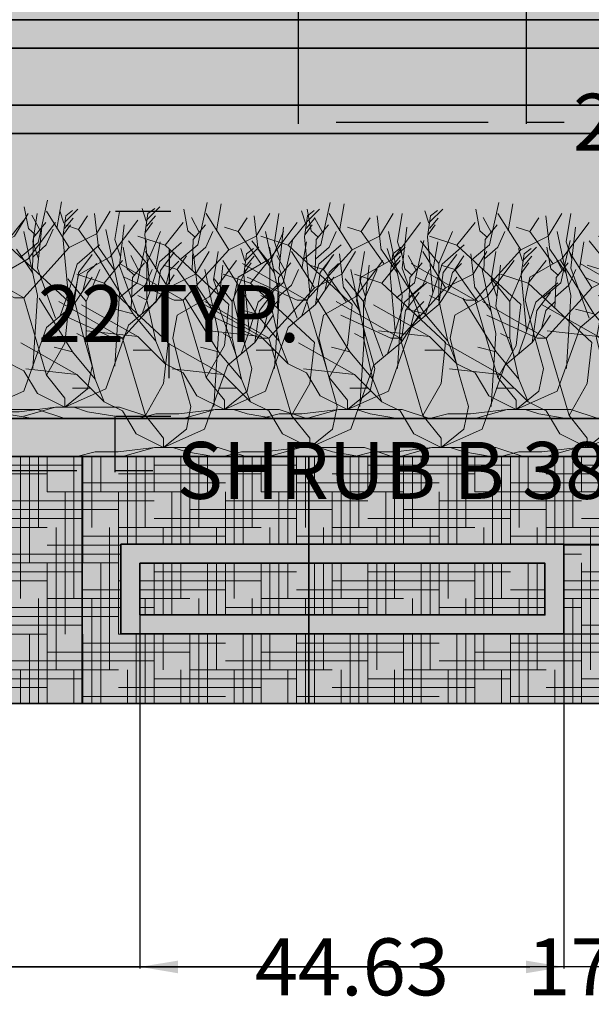
# Model space of a CAD drawing. Units: inches. Extents: x 221 to 874, y 171 to 738.
# Tile 7 of 11: x 650 to 710, y 171 to 275. Entities that reach past the tile are written whole.
import ezdxf

# ---------------------------------------------------------------- set-up
doc = ezdxf.new("R2010")
doc.units = ezdxf.units.IN
doc.header["$MEASUREMENT"] = 0
for name, color, linetype, lineweight in [('A-ANNO-DIMS', 2, 'Continuous', 18), ('A-ELEV', 7, 'Continuous', 35), ('A-ELEV-PATT', 8, 'Continuous', 13), ('L-PLNT', 3, 'Continuous', 13)]:
    doc.layers.add(name, color=color, linetype=linetype, lineweight=lineweight)
doc.styles.get("Standard").update_dxf_attribs({"font": 'arial.ttf'})
doc.dimstyles.get("Standard").update_dxf_attribs({"dimtxt": 6, "dimasz": 4, "dimexe": 0.18, "dimexo": 0.0625, "dimgap": 0.09, "dimtad": 0, "dimtih": 1, "dimtoh": 1, "dimdec": 0, "dimzin": 0, "dimdsep": 46, "dimlunit": 3, "dimtxsty": 'Standard', "dimcen": 0.09, "dimadec": 0, "dimazin": 0, "dimtfac": 1, "dimtdec": 0, "dimtofl": 0, "dimtmove": 0, "dimatfit": 3, "dimfxl": 1, "dimtolj": 1, "dimtzin": 0, "dimarcsym": 0})

# ---------------------------------------------------------------- blocks, each defined once
blk = doc.blocks.new('SHRUB-A')
for p, q in [((15.5, 17.76), (13.1, 21.6)), ((18.38, 19.2), (19.82, 21.6)), ((8.78, 18.24), (10.7, 20.64)), ((19.82, 16.8), (22.7, 20.64)), ((6.86, 16.32), (4.94, 18.72)), ((8.78, 18.24), (5.9, 19.2)), ((6.86, 16.32), (8.3, 19.68)), ((15.5, 17.76), (18.38, 19.2)), ((15.5, 12), (8.78, 18.24)), ((10.7, 12.48), (15.5, 17.76)), ((5.42, 11.04), (1.91, 16.66)), ((16.46, 14.88), (19.82, 16.8)), ((25.1, 15.36), (26.54, 17.28)), ((10.7, 12.48), (3.98, 16.32)), ((6.86, 12.48), (6.86, 16.32)), ((9.74, 12.48), (4.46, 14.88)), ((15.98, 12.48), (16.46, 14.88)), ((24.62, 12), (25.1, 15.36)), ((24.62, 12), (26.54, 14.88)), ((6.86, 12.48), (5.9, 12.96)), ((7.82, 8.16), (6.86, 12.48)), ((10.7, 12.48), (9.74, 12.48)), ((13.1, 4.32), (10.7, 12.48)), ((16.94, 8.64), (15.98, 12.48)), ((5.9, 8.64), (0, 11.96)), ((5.42, 11.04), (3.5, 11.52)), ((15.02, 7.68), (15.5, 12)), ((21.74, 9.6), (24.62, 12)), ((7.82, 8.16), (5.42, 11.04)), ((19.34, 2.88), (21.74, 9.6)), ((5.9, 8.64), (0.53, 9.22)), ((8.78, 5.76), (5.9, 8.64)), ((17.9, 5.28), (16.94, 8.64)), ((8.78, 5.76), (7.82, 8.16)), ((13.1, 4.32), (15.02, 7.68)), ((10.7, 4.8), (8.78, 5.76)), ((17.42, 2.88), (17.9, 5.28)), ((12.14, 2.4), (10.7, 4.8)), ((15.02, 1.92), (13.1, 4.32)), ((15.02, 0.96), (12.14, 2.4)), ((15.02, 0.96), (19.34, 2.88)), ((15.02, 0.96), (17.42, 2.88)), ((15.02, 0.96), (15.02, 1.92)), ((15.02, 0.96), (20.78, 0.96)), ((20.78, 0.96), (23.66, 0))]:
    blk.add_line(p, q)
blk = doc.blocks.new('GRASS-TUFT')
for p, q in [((0.28, 8.35), (0.58, 10.54)), ((0.58, 10.54), (1.31, 11.09)), ((0.83, 2.4), (0.28, 8.35)), ((1.8, 5.45), (4.12, 7.49)), ((0.83, 2.4), (1.8, 5.45)), ((0, 0), (0.83, 2.4))]:
    blk.add_line(p, q)
blk = doc.blocks.new('SHRUB-B')
for p, q in [((15.5, 17.76), (13.1, 21.6)), ((18.38, 19.2), (19.82, 21.6)), ((8.78, 18.24), (10.7, 20.64)), ((19.82, 16.8), (22.7, 20.64)), ((6.86, 16.32), (4.94, 18.72)), ((8.78, 18.24), (5.9, 19.2)), ((6.86, 16.32), (8.3, 19.68)), ((15.5, 17.76), (18.38, 19.2)), ((15.5, 12), (8.78, 18.24)), ((10.7, 12.48), (15.5, 17.76)), ((5.42, 11.04), (1.91, 16.66)), ((16.46, 14.88), (19.82, 16.8)), ((25.1, 15.36), (26.54, 17.28)), ((10.7, 12.48), (3.98, 16.32)), ((6.86, 12.48), (6.86, 16.32)), ((9.74, 12.48), (4.46, 14.88)), ((15.98, 12.48), (16.46, 14.88)), ((24.62, 12), (25.1, 15.36)), ((24.62, 12), (26.54, 14.88)), ((6.86, 12.48), (5.9, 12.96)), ((7.82, 8.16), (6.86, 12.48)), ((10.7, 12.48), (9.74, 12.48)), ((13.1, 4.32), (10.7, 12.48)), ((16.94, 8.64), (15.98, 12.48)), ((5.9, 8.64), (0, 11.96)), ((5.42, 11.04), (3.5, 11.52)), ((15.02, 7.68), (15.5, 12)), ((21.74, 9.6), (24.62, 12)), ((7.82, 8.16), (5.42, 11.04)), ((19.34, 2.88), (21.74, 9.6)), ((5.9, 8.64), (0.53, 9.22)), ((8.78, 5.76), (5.9, 8.64)), ((17.9, 5.28), (16.94, 8.64)), ((8.78, 5.76), (7.82, 8.16)), ((13.1, 4.32), (15.02, 7.68)), ((10.7, 4.8), (8.78, 5.76)), ((17.42, 2.88), (17.9, 5.28)), ((12.14, 2.4), (10.7, 4.8)), ((15.02, 1.92), (13.1, 4.32)), ((15.02, 0.96), (12.14, 2.4)), ((15.02, 0.96), (19.34, 2.88)), ((15.02, 0.96), (17.42, 2.88)), ((15.02, 0.96), (15.02, 1.92)), ((15.02, 0.96), (20.78, 0.96)), ((20.78, 0.96), (23.66, 0)), ((25.58, 0.48), (23.66, 0)), ((27.98, 0.48), (25.58, 0.48)), ((31.82, 0.96), (27.98, 0.48)), ((31.82, 0.96), (28.46, 0)), ((31.82, 0.96), (33.74, 0.96)), ((33.74, 0.96), (35.18, 0.48)), ((35.18, 0.48), (38.06, 0))]:
    blk.add_line(p, q)
blk = doc.blocks.new('GRASS-SPRIG')
for p, q in [((1.44, 3.36), (2.4, 4.8)), ((1.44, 3.36), (0, 3.84)), ((3.84, 0), (1.44, 3.36))]:
    blk.add_line(p, q)
blk = doc.blocks.new('*D13')
at = {"layer": 'A-ANNO-DIMS', "color": 0, "lineweight": -2, "transparency": 16777216}
for p, q in [((678.91, 283.65), (678.91, 263.74)), ((702.91, 283.65), (702.91, 263.74)), ((682.91, 263.92), (698.91, 263.92)), ((702.91, 263.92), (706.91, 263.92))]:
    blk.add_line(p, q, dxfattribs=at)
at = {"layer": 'A-ANNO-DIMS', "color": 0, "transparency": 16777216}
for points in [[(682.91, 264.58), (682.91, 263.25), (678.91, 263.92)], [(698.91, 264.58), (698.91, 263.25), (702.91, 263.92)]]:
    blk.add_solid(points, dxfattribs=at)
at = {"layer": 'Defpoints', "color": 0, "transparency": 16777216}
for p in [(678.91, 283.72), (702.91, 283.72), (702.91, 263.92)]:
    blk.add_point(p, dxfattribs=at)
at = {"layer": 'A-ANNO-DIMS', "color": 0, "transparency": 16777216, "insert": (721.65, 263.92), "char_height": 6, "attachment_point": 5}
blk.add_mtext('\\A1;24 TYP.', dxfattribs=at)
blk = doc.blocks.new('*D16')
at = {"layer": 'A-ANNO-DIMS', "color": 0, "lineweight": -2, "transparency": 16777216}
for p, q in [((621.56, 232.89), (621.56, 227.07)), ((659.62, 232.89), (659.62, 227.07)), ((625.56, 227.25), (655.62, 227.25)), ((659.62, 227.25), (663.62, 227.25))]:
    blk.add_line(p, q, dxfattribs=at)
at = {"layer": 'A-ANNO-DIMS', "color": 0, "transparency": 16777216}
for points in [[(625.56, 227.91), (625.56, 226.58), (621.56, 227.25)], [(655.62, 227.91), (655.62, 226.58), (659.62, 227.25)]]:
    blk.add_solid(points, dxfattribs=at)
at = {"layer": 'Defpoints', "color": 0, "transparency": 16777216}
for p in [(621.56, 232.96), (659.62, 232.96), (659.62, 227.25)]:
    blk.add_point(p, dxfattribs=at)
at = {"layer": 'A-ANNO-DIMS', "color": 0, "transparency": 16777216, "insert": (698.1, 227.25), "char_height": 6, "attachment_point": 5}
blk.add_mtext('\\A1;SHRUB B 38 TYP.', dxfattribs=at)
blk = doc.blocks.new('*D17')
at = {"layer": 'A-ANNO-DIMS', "color": 0, "lineweight": -2, "transparency": 16777216}
for p, q in [((659.69, 254.56), (665.51, 254.56)), ((665.33, 250.56), (665.33, 246.86)), ((665.33, 236.96), (665.33, 240.65)), ((659.69, 232.96), (665.51, 232.96))]:
    blk.add_line(p, q, dxfattribs=at)
at = {"layer": 'A-ANNO-DIMS', "color": 0, "transparency": 16777216}
for points in [[(664.67, 250.56), (666, 250.56), (665.33, 254.56)], [(664.67, 236.96), (666, 236.96), (665.33, 232.96)]]:
    blk.add_solid(points, dxfattribs=at)
at = {"layer": 'Defpoints', "color": 0, "transparency": 16777216}
for p in [(659.62, 254.56), (665.33, 254.56), (659.62, 232.96)]:
    blk.add_point(p, dxfattribs=at)
at = {"layer": 'A-ANNO-DIMS', "color": 0, "transparency": 16777216, "insert": (665.33, 243.76), "char_height": 6, "attachment_point": 5}
blk.add_mtext('\\A1;22 TYP.', dxfattribs=at)
blk = doc.blocks.new('*D20')
at = {"layer": 'A-ANNO-DIMS', "color": 0, "lineweight": -2, "transparency": 16777216}
for p, q in [((313.08, 202.65), (313.08, 174.79)), ((805.08, 202.65), (805.08, 174.79)), ((317.08, 174.97), (552.27, 174.97)), ((801.08, 174.97), (565.89, 174.97))]:
    blk.add_line(p, q, dxfattribs=at)
at = {"layer": 'A-ANNO-DIMS', "color": 0, "transparency": 16777216}
for points in [[(317.08, 175.63), (317.08, 174.3), (313.08, 174.97)], [(801.08, 175.63), (801.08, 174.3), (805.08, 174.97)]]:
    blk.add_solid(points, dxfattribs=at)
at = {"layer": 'Defpoints', "color": 0, "transparency": 16777216}
for p in [(313.08, 202.72), (805.08, 202.72), (805.08, 174.97)]:
    blk.add_point(p, dxfattribs=at)
at = {"layer": 'A-ANNO-DIMS', "color": 0, "transparency": 16777216, "insert": (559.08, 174.97), "char_height": 6, "attachment_point": 5}
blk.add_mtext('\\A1;492', dxfattribs=at)
blk = doc.blocks.new('*D21')
at = {"layer": 'A-ANNO-DIMS', "color": 0, "lineweight": -2, "transparency": 16777216}
for p, q in [((541.14, 706.72), (833.01, 706.72)), ((832.83, 702.72), (832.83, 457.87)), ((832.83, 206.72), (832.83, 451.56)), ((805.14, 202.72), (833.01, 202.72))]:
    blk.add_line(p, q, dxfattribs=at)
at = {"layer": 'A-ANNO-DIMS', "color": 0, "transparency": 16777216}
for points in [[(832.16, 702.72), (833.5, 702.72), (832.83, 706.72)], [(832.16, 206.72), (833.5, 206.72), (832.83, 202.72)]]:
    blk.add_solid(points, dxfattribs=at)
at = {"layer": 'Defpoints', "color": 0, "transparency": 16777216}
for p in [(541.08, 706.72), (832.83, 706.72), (805.08, 202.72)]:
    blk.add_point(p, dxfattribs=at)
at = {"layer": 'A-ANNO-DIMS', "color": 0, "transparency": 16777216, "insert": (832.83, 454.72), "char_height": 6, "attachment_point": 5}
blk.add_mtext('\\A1;504', dxfattribs=at)
blk = doc.blocks.new('*D64')
at = {"layer": 'A-ANNO-DIMS', "color": 0, "lineweight": -2, "transparency": 16777216}
for p, q in [((832.83, 284.72), (832.83, 288.72)), ((832.83, 288.72), (836.83, 288.72)), ((705.97, 280.72), (833.01, 280.72)), ((781.14, 274.72), (833.01, 274.72)), ((832.83, 270.72), (832.83, 266.72))]:
    blk.add_line(p, q, dxfattribs=at)
at = {"layer": 'A-ANNO-DIMS', "color": 0, "transparency": 16777216}
for points in [[(832.16, 284.72), (833.5, 284.72), (832.83, 280.72)], [(832.16, 270.72), (833.5, 270.72), (832.83, 274.72)]]:
    blk.add_solid(points, dxfattribs=at)
at = {"layer": 'Defpoints', "color": 0, "transparency": 16777216}
for p in [(705.91, 280.72), (832.83, 280.72), (781.08, 274.72)]:
    blk.add_point(p, dxfattribs=at)
at = {"layer": 'A-ANNO-DIMS', "color": 0, "transparency": 16777216, "insert": (838.9, 288.72), "char_height": 6, "attachment_point": 5}
blk.add_mtext('\\A1;6', dxfattribs=at)
blk = doc.blocks.new('*D70')
at = {"layer": 'A-ANNO-DIMS', "color": 0, "lineweight": -2, "transparency": 16777216}
for p, q in [((625.96, 229.65), (625.96, 174.79)), ((805.08, 202.65), (805.08, 174.79)), ((629.96, 174.97), (703.29, 174.97)), ((801.08, 174.97), (727.75, 174.97))]:
    blk.add_line(p, q, dxfattribs=at)
at = {"layer": 'A-ANNO-DIMS', "color": 0, "transparency": 16777216}
for points in [[(629.96, 175.63), (629.96, 174.3), (625.96, 174.97)], [(801.08, 175.63), (801.08, 174.3), (805.08, 174.97)]]:
    blk.add_solid(points, dxfattribs=at)
at = {"layer": 'Defpoints', "color": 0, "transparency": 16777216}
for p in [(625.96, 229.72), (805.08, 202.72), (805.08, 174.97)]:
    blk.add_point(p, dxfattribs=at)
at = {"layer": 'A-ANNO-DIMS', "color": 0, "transparency": 16777216, "insert": (715.52, 174.97), "char_height": 6, "attachment_point": 5}
blk.add_mtext('\\A1;179.12', dxfattribs=at)
blk = doc.blocks.new('*D71')
at = {"layer": 'A-ANNO-DIMS', "color": 0, "lineweight": -2, "transparency": 16777216}
for p, q in [((662.26, 211.97), (662.26, 174.79)), ((706.89, 209.97), (706.89, 174.79)), ((666.26, 174.97), (674.24, 174.97)), ((702.89, 174.97), (694.91, 174.97))]:
    blk.add_line(p, q, dxfattribs=at)
at = {"layer": 'A-ANNO-DIMS', "color": 0, "transparency": 16777216}
for points in [[(666.26, 175.63), (666.26, 174.3), (662.26, 174.97)], [(702.89, 175.63), (702.89, 174.3), (706.89, 174.97)]]:
    blk.add_solid(points, dxfattribs=at)
at = {"layer": 'Defpoints', "color": 0, "transparency": 16777216}
for p in [(662.26, 212.04), (706.89, 210.04), (706.89, 174.97)]:
    blk.add_point(p, dxfattribs=at)
at = {"layer": 'A-ANNO-DIMS', "color": 0, "transparency": 16777216, "insert": (684.57, 174.97), "char_height": 6, "attachment_point": 5}
blk.add_mtext('\\A1;44.63', dxfattribs=at)
blk = doc.blocks.new('*D72')
at = {"layer": 'A-ANNO-DIMS', "color": 0, "lineweight": -2, "transparency": 16777216}
for p, q in [((832.83, 219.48), (832.83, 223.48)), ((832.83, 223.48), (836.83, 223.48)), ((706.95, 219.48), (833.01, 219.48)), ((832.83, 214.04), (832.83, 215.48)), ((706.95, 210.04), (833.01, 210.04))]:
    blk.add_line(p, q, dxfattribs=at)
at = {"layer": 'A-ANNO-DIMS', "color": 0, "transparency": 16777216}
for points in [[(832.16, 215.48), (833.5, 215.48), (832.83, 219.48)], [(832.16, 214.04), (833.5, 214.04), (832.83, 210.04)]]:
    blk.add_solid(points, dxfattribs=at)
at = {"layer": 'Defpoints', "color": 0, "transparency": 16777216}
for p in [(706.89, 219.48), (832.83, 219.48), (706.89, 210.04)]:
    blk.add_point(p, dxfattribs=at)
at = {"layer": 'A-ANNO-DIMS', "color": 0, "transparency": 16777216, "insert": (847.03, 223.48), "char_height": 6, "attachment_point": 5}
blk.add_mtext('\\A1;9.444', dxfattribs=at)

msp = doc.modelspace()

# ---------------------------------------------------------------- hatches: boundary and pattern name
at = {"layer": 'A-ELEV-PATT'}
h = msp.add_hatch(color=256, dxfattribs=at)
h.dxf.hatch_style = 1
h.paths.add_polyline_path([(349.0786, 286.1996), (313.0786, 286.1996), (313.0786, 232.7164), (349.0786, 232.7164)])
h.paths.add_polyline_path([(464.0786, 286.1996), (406.0786, 286.1996), (406.0786, 232.7164), (464.0786, 232.7164)])
h.paths.add_polyline_path([(541.0786, 286.1996), (493.0786, 286.1996), (493.0786, 232.7164), (541.0786, 232.7164)])
h.paths.add_polyline_path([(541.0786, 370.7164), (493.0786, 370.7164), (493.0786, 286.1996), (541.0786, 286.1996)])
h.paths.add_polyline_path([(464.0786, 370.7164), (406.0786, 370.7164), (406.0786, 286.1996), (464.0786, 286.1996)])
h.paths.add_polyline_path([(349.0786, 370.7164), (313.0786, 370.7164), (313.0786, 286.1996), (349.0786, 286.1996)])
h.paths.add_polyline_path([(349.0786, 454.7164), (313.0786, 454.7164), (313.0786, 370.7164), (349.0786, 370.7164)])
h.paths.add_polyline_path([(464.0786, 454.7164), (406.0786, 454.7164), (406.0786, 370.7164), (464.0786, 370.7164)])
h.paths.add_polyline_path([(541.0786, 418.7164), (541.0786, 454.7164), (493.0786, 454.7164), (493.0786, 370.7164), (541.0786, 370.7164)])
h.paths.add_polyline_path([(541.0786, 550.7164), (493.0786, 550.7164), (493.0786, 454.7164), (541.0786, 454.7164)])
h.paths.add_polyline_path([(464.0786, 550.7164), (406.0786, 550.7164), (406.0786, 454.7164), (464.0786, 454.7164)])
h.paths.add_polyline_path([(349.0786, 550.7164), (313.0786, 550.7164), (313.0786, 454.7164), (349.0786, 454.7164)])
h.paths.add_polyline_path([(349.0786, 586.7164), (313.0786, 586.7164), (313.0786, 550.7164), (349.0786, 550.7164)])
h.paths.add_polyline_path([(464.0786, 586.7164), (406.0786, 586.7164), (406.0786, 550.7164), (464.0786, 550.7164)])
h.paths.add_polyline_path([(541.0786, 574.7164), (541.0786, 586.7164), (493.0786, 586.7164), (493.0786, 550.7164), (541.0786, 550.7164)])
h.paths.add_polyline_path([(541.0786, 670.7164), (493.0786, 670.7164), (493.0786, 586.7164), (541.0786, 586.7164)])
h.paths.add_polyline_path([(464.0786, 670.7164), (406.0786, 670.7164), (406.0786, 586.7164), (464.0786, 586.7164)])
h.paths.add_polyline_path([(349.0786, 670.7164), (313.0786, 670.7164), (313.0786, 586.7164), (349.0786, 586.7164)])
h.paths.add_polyline_path([(406.0786, 706.7164), (313.0786, 706.7164), (313.0786, 670.7164), (349.0786, 670.7164), (406.0786, 670.7164)])
h.paths.add_polyline_path([(464.0786, 706.7164), (406.0786, 706.7164), (406.0786, 670.7164), (464.0786, 670.7164)])
h.paths.add_polyline_path([(541.0786, 706.7164), (493.0786, 706.7164), (493.0786, 688.7164), (493.0786, 670.7164), (541.0786, 670.7164)])
h.paths.add_polyline_path([(660.0786, 610.7164), (541.0786, 610.7164), (541.0786, 586.7164), (541.0786, 574.7164), (660.0786, 574.7164)])
h.paths.add_polyline_path([(781.0786, 610.7164), (660.0786, 610.7164), (660.0786, 574.7164), (769.0786, 574.7164), (781.0786, 574.7164)])
h.paths.add_polyline_path([(781.0786, 574.7164), (769.0786, 574.7164), (769.0786, 476.1199), (781.0786, 476.1199)])
h.paths.add_polyline_path([(781.0786, 476.1199), (769.0786, 476.1199), (769.0786, 457.7164), (781.0786, 457.7164)])
h.paths.add_polyline_path([(781.0786, 377.1023), (705.9097, 377.1023), (705.9097, 286.1996), (781.0786, 286.1996)])
h.paths.add_polyline_path([(741.9618, 338.8486), (756.9618, 338.8486), (756.9618, 329.8486), (741.9618, 329.8486)], flags=16)
h.paths.add_polyline_path([(648.9097, 377.1023), (598.0786, 377.1023), (598.0786, 286.1996), (648.9097, 286.1996)])
h.paths.add_polyline_path([(781.0786, 286.1996), (705.9097, 286.1996), (705.9097, 280.7164), (648.9097, 280.7164), (648.9097, 286.1996), (598.0786, 286.1996), (598.0786, 280.7164), (550.0786, 280.7164), (550.0786, 286.1996), (541.0786, 286.1996), (541.0786, 274.7164), (781.0786, 274.7164)])
h.paths.add_polyline_path([(660.0786, 562.7164), (546.3477, 562.7164), (546.3477, 457.7164), (660.0786, 457.7164)])
h = msp.add_hatch(color=256, dxfattribs=at)
h.set_gradient(color1=(99, 100, 102), color2=(169, 160, 132), name='INVCYLINDER')
h.paths.add_polyline_path([(541.0786, 274.7164), (541.0786, 271.7164), (787.0786, 271.7164), (781.0786, 274.7164)])
h = msp.add_hatch(color=256, dxfattribs=at)
h.paths.add_polyline_path([(787.0786, 271.7164), (541.0786, 271.7164), (541.0786, 265.7164), (799.0786, 265.7164)])
h.paths.add_polyline_path([(631.9596, 262.7164), (541.0786, 262.7164), (541.0786, 256.7164), (631.9596, 256.7164)])
h.paths.add_polyline_path([(631.9596, 253.7164), (541.0786, 253.7164), (541.0786, 247.7164), (631.9596, 247.7164)])
h.paths.add_polyline_path([(631.9596, 244.7164), (541.0786, 244.7164), (541.0786, 238.7164), (631.9596, 238.7164)])
h.paths.add_polyline_path([(631.9596, 235.7164), (541.0786, 235.7164), (541.0786, 229.7164), (625.9596, 229.7164), (625.9596, 232.7164), (631.9596, 232.7164)])
h.paths.add_polyline_path([(630.2472, 217.7164), (538.2859, 217.7164), (538.2859, 211.7164), (634.5124, 211.7164), (634.5123, 211.7326)], flags=17)
h.paths.add_polyline_path([(634.5396, 208.7164), (538.2859, 208.7164), (538.2859, 202.7164), (638.8162, 202.7164)])
h = msp.add_hatch(color=256, dxfattribs=at)
h.set_gradient(color1=(99, 100, 102), color2=(248, 246, 176), name='CYLINDER')
h.paths.add_polyline_path([(805.0786, 262.7164), (799.0786, 265.7164), (541.0786, 265.7164), (541.0786, 262.7164)])
for points in [[(631.9596, 262.7164), (631.9596, 232.7164), (805.0786, 232.7164), (805.0786, 262.7164)], [(805.0786, 228.7164), (805.0786, 232.7164), (625.9596, 232.7164), (625.9596, 228.7164)]]:
    msp.add_hatch(color=256, dxfattribs=at).paths.add_polyline_path(points)
h = msp.add_hatch(color=256, dxfattribs=at)
h.set_gradient(color1=(147, 149, 152), color2=(99, 100, 102), name='CURVED')
h.paths.add_polyline_path([(656.1863, 228.7164), (625.9606, 228.7164), (625.9626, 226.7164), (630.2279, 220.7164), (630.2471, 217.7164), (634.5238, 211.7164), (634.5124, 211.7164), (634.5315, 208.7276), (638.8162, 202.7164), (656.1863, 202.7164)])
h = msp.add_hatch(dxfattribs=at)
h.set_pattern_fill('HOUND', color=256, scale=15, style=0)
h.paths.add_polyline_path([(656.1863, 228.7164), (625.9606, 228.7164), (625.9626, 226.7164), (630.2279, 220.7164), (630.2471, 217.7164), (634.5238, 211.7164), (634.5124, 211.7164), (634.5315, 208.7276), (638.8162, 202.7164), (656.1863, 202.7164)])
h = msp.add_hatch(color=256, dxfattribs=at)
h.set_gradient(color1=(99, 100, 102), color2=(91, 91, 91), rotation=180, name='INVCURVED')
h.paths.add_polyline_path([(680.047, 219.4807), (680.047, 228.7164), (656.1863, 228.7164), (656.1863, 202.7164), (680.047, 202.7164), (680.047, 210.037), (660.2585, 210.037), (660.2585, 219.4807)])
h.paths.add_polyline_path([(662.2585, 217.4807), (662.2585, 212.037), (680.047, 212.037), (680.047, 217.4807)], flags=17)
h.paths.add_polyline_path([(782.8632, 202.7164), (782.8632, 228.7164), (735.4784, 228.7164), (735.4784, 202.7164)])
h = msp.add_hatch(dxfattribs=at)
h.set_pattern_fill('HOUND', color=256, scale=15, style=0)
h.paths.add_polyline_path([(680.047, 228.7164), (656.1863, 228.7164), (656.1863, 202.7164), (680.047, 202.7164), (680.047, 210.037), (660.2585, 210.037), (660.2585, 219.4807), (680.047, 219.4807)])
h.paths.add_polyline_path([(680.047, 217.4807), (662.2585, 217.4807), (662.2585, 212.037), (680.047, 212.037)], flags=17)
h = msp.add_hatch(color=256, dxfattribs=at)
h.set_gradient(color1=(147, 149, 152), color2=(99, 100, 102), name='CURVED')
h.paths.add_polyline_path([(735.4784, 202.7164), (735.4784, 228.7164), (680.047, 228.7164), (680.047, 219.4807), (706.8876, 219.4807), (706.8876, 210.037), (680.047, 210.037), (680.047, 202.7164)])
h.paths.add_polyline_path([(680.047, 217.4807), (680.047, 212.037), (704.8876, 212.037), (704.8876, 217.4807)], flags=17)
h = msp.add_hatch(dxfattribs=at)
h.set_pattern_fill('HOUND', color=256, scale=15, style=0)
h.paths.add_polyline_path([(735.4784, 228.7164), (680.047, 228.7164), (680.047, 219.4807), (706.8876, 219.4807), (706.8876, 210.037), (680.047, 210.037), (680.047, 202.7164), (735.4784, 202.7164)])
h.paths.add_polyline_path([(704.8876, 217.4807), (680.047, 217.4807), (680.047, 212.037), (704.8876, 212.037)], flags=17)
h = msp.add_hatch(color=256, dxfattribs=at)
h.paths.add_polyline_path([(706.8876, 219.4807), (660.2585, 219.4807), (660.2585, 210.037), (706.8876, 210.037)])
h.paths.add_polyline_path([(704.8876, 217.4807), (704.8876, 212.037), (662.2585, 212.037), (662.2585, 217.4807)], flags=16)

# ---------------------------------------------------------------- linework, layer by layer
at = {"layer": 'A-ELEV'}
for p, q in [((781.0786, 274.7164), (541.0786, 274.7164)), ((787.0786, 271.7164), (541.0786, 271.7164)), ((799.0786, 265.7164), (541.0786, 265.7164)), ((805.0786, 262.7164), (541.0786, 262.7164)), ((805.0786, 232.7164), (625.9596, 232.7164)), ((805.0786, 228.7164), (625.9596, 228.7164)), ((656.1863, 202.7164), (656.1863, 228.7164)), ((680.047, 202.7164), (680.047, 228.7164)), ((805.0786, 202.7164), (313.0786, 202.7164))]:
    msp.add_line(p, q, dxfattribs=at)
for points in [[(660.2585, 219.4807), (706.8876, 219.4807), (706.8876, 210.037), (660.2585, 210.037)], [(662.2585, 217.4807), (704.8876, 217.4807), (704.8876, 212.037), (662.2585, 212.037)]]:
    msp.add_lwpolyline(points, close=True, dxfattribs=at)
at = {"layer": 'L-PLNT'}
for p, q in [((651.5505, 251.2454), (652.5265, 255.7054)), ((653.5035, 252.7314), (653.9915, 255.5484)), ((668.3505, 251.0054), (669.3265, 255.4654)), ((670.3035, 252.4914), (670.7915, 255.3084)), ((681.3105, 251.0054), (682.2865, 255.4654)), ((683.2635, 252.4914), (683.7515, 255.3084)), ((699.0705, 251.0054), (700.0465, 255.4654)), ((701.0235, 252.4914), (701.5115, 255.3084)), ((650.5125, 252.7314), (650.0855, 255.0004)), ((651.7035, 252.5754), (650.8795, 254.1404)), ((650.9665, 251.3184), (651.4555, 254.2914)), ((653.8355, 254.6044), (654.2625, 253.2744)), ((654.3845, 253.4304), (655.7275, 254.7604)), ((657.8975, 250.6974), (657.4705, 254.2964)), ((659.6065, 251.5584), (660.0955, 254.5314)), ((662.4755, 254.8444), (662.9025, 253.5144)), ((662.9635, 252.9664), (663.8795, 254.0614)), ((663.0245, 253.6704), (664.3675, 255.0004)), ((667.3125, 252.4914), (666.8855, 254.7604)), ((671.6235, 250.4764), (669.2235, 254.3164)), ((674.6975, 250.4574), (674.2705, 254.0564)), ((674.5035, 251.9164), (675.9435, 254.3164)), ((676.4065, 251.3184), (676.8955, 254.2914)), ((679.2755, 254.6044), (679.7025, 253.2744)), ((679.8245, 253.4304), (681.1675, 254.7604)), ((680.2725, 252.4914), (679.8455, 254.7604)), ((684.5835, 250.4764), (682.1835, 254.3164)), ((687.6575, 250.4574), (687.2305, 254.0564)), ((687.4635, 251.9164), (688.9035, 254.3164)), ((689.3665, 251.3184), (689.8555, 254.2914)), ((692.2355, 254.6044), (692.6625, 253.2744)), ((692.7845, 253.4304), (694.1275, 254.7604)), ((698.0325, 252.4914), (697.6055, 254.7604)), ((702.3435, 250.4764), (699.9435, 254.3164)), ((705.4175, 250.4574), (704.9905, 254.0564)), ((705.2235, 251.9164), (706.6635, 254.3164)), ((707.1265, 251.3184), (707.6155, 254.2914)), ((651.0625, 251.7924), (652.3435, 253.3574)), ((654.2015, 252.1004), (654.9335, 253.1174)), ((654.3235, 252.7264), (655.2395, 253.8214)), ((660.1035, 248.7964), (660.5835, 253.1164)), ((662.8415, 252.3404), (663.5735, 253.3574)), ((664.9035, 250.9564), (666.8235, 253.3564)), ((668.5035, 252.3354), (667.6795, 253.9004)), ((667.8625, 251.5524), (669.1435, 253.1174)), ((675.9435, 249.5164), (678.8235, 253.3564)), ((677.8635, 250.9564), (679.7835, 253.3564)), ((679.6415, 252.1004), (680.3735, 253.1174)), ((679.7635, 252.7264), (680.6795, 253.8214)), ((681.4635, 252.3354), (680.6395, 253.9004)), ((680.8225, 251.5524), (682.1035, 253.1174)), ((688.9035, 249.5164), (691.7835, 253.3564)), ((692.6015, 252.1004), (693.3335, 253.1174)), ((692.7235, 252.7264), (693.6395, 253.8214)), ((695.6235, 250.9564), (697.5435, 253.3564)), ((699.2235, 252.3354), (698.3995, 253.9004)), ((698.5825, 251.5524), (699.8635, 253.1174)), ((706.6635, 249.5164), (709.5435, 253.3564)), ((651.4635, 245.6764), (650.0235, 252.3964)), ((651.3065, 252.0274), (650.5125, 252.7314)), ((651.4635, 248.5564), (651.9435, 252.8764)), ((652.4045, 251.0104), (653.1375, 252.6534)), ((660.1035, 245.9164), (658.6635, 252.6364)), ((662.9835, 249.0364), (664.4235, 252.3964)), ((668.1065, 251.7874), (667.3125, 252.4914)), ((669.2045, 250.7704), (669.9375, 252.4134)), ((676.9035, 245.6764), (675.4635, 252.3964)), ((675.9435, 249.0364), (677.3835, 252.3964)), ((676.9035, 248.5564), (677.3835, 252.8764)), ((681.0665, 251.7874), (680.2725, 252.4914)), ((682.1645, 250.7704), (682.8975, 252.4134)), ((689.8635, 245.6764), (688.4235, 252.3964)), ((689.8635, 248.5564), (690.3435, 252.8764)), ((693.7035, 249.0364), (695.1435, 252.3964)), ((698.8265, 251.7874), (698.0325, 252.4914)), ((699.9245, 250.7704), (700.6575, 252.4134)), ((707.6235, 245.6764), (706.1835, 252.3964)), ((707.6235, 248.5564), (708.1035, 252.8764)), ((649.6585, 249.6804), (651.5505, 251.2454)), ((650.9405, 248.5844), (651.0625, 251.7924)), ((651.5775, 249.5184), (650.9665, 251.3184)), ((651.0015, 249.7584), (652.4045, 251.0104)), ((660.2175, 249.7584), (659.6065, 251.5584)), ((662.9835, 249.0364), (661.0635, 251.4364)), ((661.9584, 247.0054), (662.9344, 251.4654)), ((664.9035, 250.9564), (662.0235, 251.9164)), ((663.9114, 248.4914), (664.3994, 251.3084)), ((671.6235, 244.7164), (664.9035, 250.9564)), ((666.4585, 249.4404), (668.3505, 251.0054)), ((667.7405, 248.3444), (667.8625, 251.5524)), ((671.6235, 250.4764), (674.5035, 251.9164)), ((675.9435, 249.0364), (674.0235, 251.4364)), ((677.8635, 250.9564), (674.9835, 251.9164)), ((677.0175, 249.5184), (676.4065, 251.3184)), ((677.3482, 247.0054), (678.3242, 251.4654)), ((684.5835, 244.7164), (677.8635, 250.9564)), ((679.3012, 248.4914), (679.7892, 251.3084)), ((679.4185, 249.4404), (681.3105, 251.0054)), ((680.7005, 248.3444), (680.8225, 251.5524)), ((684.5835, 250.4764), (687.4635, 251.9164)), ((689.9775, 249.5184), (689.3665, 251.3184)), ((691.1676, 247.0054), (692.1436, 251.4654)), ((693.7035, 249.0364), (691.7835, 251.4364)), ((695.6235, 250.9564), (692.7435, 251.9164)), ((693.1206, 248.4914), (693.6086, 251.3084)), ((702.3435, 244.7164), (695.6235, 250.9564)), ((697.1785, 249.4404), (699.0705, 251.0054)), ((698.4605, 248.3444), (698.5825, 251.5524)), ((702.3435, 250.4764), (705.2235, 251.9164)), ((706.5574, 247.0054), (707.5334, 251.4654)), ((707.7375, 249.5184), (707.1265, 251.3184)), ((708.5104, 248.4914), (708.9984, 251.3084)), ((650.9665, 248.0314), (649.2575, 250.5354)), ((659.6065, 248.2714), (657.8975, 250.7754)), ((660.9204, 248.4914), (660.4934, 250.7604)), ((662.1114, 248.3354), (661.2874, 249.9004)), ((666.8235, 245.1964), (671.6235, 250.4764)), ((667.8015, 249.5184), (669.2045, 250.7704)), ((668.3054, 246.4574), (667.8784, 250.0564)), ((670.0144, 247.3184), (670.5034, 250.2914)), ((672.8834, 250.6044), (673.3104, 249.2744)), ((673.4324, 249.4304), (674.7754, 250.7604)), ((676.4065, 248.0314), (674.6975, 250.5354)), ((676.3102, 248.4914), (675.8832, 250.7604)), ((677.5012, 248.3354), (676.6772, 249.9004)), ((679.7835, 245.1964), (684.5835, 250.4764)), ((680.7615, 249.5184), (682.1645, 250.7704)), ((681.2235, 248.0764), (682.6635, 249.9964)), ((683.6952, 246.4574), (683.2682, 250.0564)), ((685.4042, 247.3184), (685.8932, 250.2914)), ((689.3665, 248.0314), (687.6575, 250.5354)), ((688.2732, 250.6044), (688.7002, 249.2744)), ((688.8222, 249.4304), (690.1652, 250.7604)), ((690.1296, 248.4914), (689.7026, 250.7604)), ((691.3206, 248.3354), (690.4966, 249.9004)), ((694.1835, 248.0764), (695.6235, 249.9964)), ((697.5146, 246.4574), (697.0876, 250.0564)), ((697.5435, 245.1964), (702.3435, 250.4764)), ((698.5215, 249.5184), (699.9245, 250.7704)), ((699.2236, 247.3184), (699.7126, 250.2914)), ((702.0926, 250.6044), (702.5196, 249.2744)), ((702.6416, 249.4304), (703.9846, 250.7604)), ((705.5194, 248.4914), (705.0924, 250.7604)), ((707.1265, 248.0314), (705.4175, 250.5354)), ((706.7104, 248.3354), (705.8864, 249.9004)), ((656.7435, 248.0764), (657.7035, 249.0364)), ((661.5435, 243.7564), (658.0285, 249.3714)), ((666.8235, 245.1964), (660.1035, 249.0364)), ((661.4704, 247.5524), (662.7514, 249.1174)), ((662.9835, 245.1964), (662.9835, 249.0364)), ((665.3835, 248.3164), (666.3435, 249.2764)), ((670.5114, 244.5564), (670.9914, 248.8764)), ((674.5035, 243.7564), (670.9885, 249.3714)), ((672.5835, 247.5964), (675.9435, 249.5164)), ((679.7835, 245.1964), (673.0635, 249.0364)), ((673.2494, 248.1004), (673.9814, 249.1174)), ((673.3714, 248.7264), (674.2874, 249.8214)), ((675.9435, 245.1964), (675.9435, 249.0364)), ((676.8602, 247.5524), (678.1412, 249.1174)), ((682.1835, 248.0764), (683.1435, 249.0364)), ((685.5435, 247.5964), (688.9035, 249.5164)), ((685.9012, 244.5564), (686.3812, 248.8764)), ((688.6392, 248.1004), (689.3712, 249.1174)), ((692.2635, 243.7564), (688.7485, 249.3714)), ((688.7612, 248.7264), (689.6772, 249.8214)), ((690.6796, 247.5524), (691.9606, 249.1174)), ((697.5435, 245.1964), (690.8235, 249.0364)), ((693.7035, 245.1964), (693.7035, 249.0364)), ((695.1435, 248.0764), (696.1035, 249.0364)), ((699.7206, 244.5564), (700.2006, 248.8764)), ((702.4586, 248.1004), (703.1906, 249.1174)), ((702.5806, 248.7264), (703.4966, 249.8214)), ((703.3035, 247.5964), (706.6635, 249.5164)), ((706.0694, 247.5524), (707.3504, 249.1174)), ((653.3835, 243.2764), (651.4635, 248.5564)), ((656.2635, 246.1564), (656.7435, 248.0764)), ((662.0235, 243.5164), (660.1035, 248.7964)), ((661.7144, 247.7874), (660.9204, 248.4914)), ((662.8124, 246.7704), (663.5454, 248.4134)), ((664.9035, 246.3964), (665.3835, 248.3164)), ((670.5114, 241.6764), (669.0714, 248.3964)), ((677.1042, 247.7874), (676.3102, 248.4914)), ((678.8235, 243.2764), (676.9035, 248.5564)), ((678.2022, 246.7704), (678.9352, 248.4134)), ((680.7435, 244.7164), (681.2235, 248.0764)), ((681.7035, 246.1564), (682.1835, 248.0764)), ((685.9012, 241.6764), (684.4612, 248.3964)), ((691.7835, 243.2764), (689.8635, 248.5564)), ((690.9236, 247.7874), (690.1296, 248.4914)), ((692.0216, 246.7704), (692.7546, 248.4134)), ((693.7035, 244.7164), (694.1835, 248.0764)), ((694.6635, 246.1564), (695.1435, 248.0764)), ((699.7206, 241.6764), (698.2806, 248.3964)), ((706.3134, 247.7874), (705.5194, 248.4914)), ((707.4114, 246.7704), (708.1444, 248.4134)), ((709.5435, 243.2764), (707.6235, 248.5564)), ((660.0664, 245.4404), (661.9584, 247.0054)), ((665.8635, 245.1964), (660.5835, 247.5964)), ((661.3484, 244.3444), (661.4704, 247.5524)), ((670.6254, 245.5184), (670.0144, 247.3184)), ((672.1035, 245.1964), (672.5835, 247.5964)), ((678.8235, 245.1964), (673.5435, 247.5964)), ((675.4562, 245.4404), (677.3482, 247.0054)), ((676.7382, 244.3444), (676.8602, 247.5524)), ((680.7435, 244.7164), (682.6635, 247.5964)), ((685.0635, 245.1964), (685.5435, 247.5964)), ((686.0152, 245.5184), (685.4042, 247.3184)), ((689.2756, 245.4404), (691.1676, 247.0054)), ((690.5576, 244.3444), (690.6796, 247.5524)), ((696.5835, 245.1964), (691.3035, 247.5964)), ((693.7035, 244.7164), (695.6235, 247.5964)), ((699.8346, 245.5184), (699.2236, 247.3184)), ((702.8235, 245.1964), (703.3035, 247.5964)), ((704.6654, 245.4404), (706.5574, 247.0054)), ((705.9474, 244.3444), (706.0694, 247.5524)), ((659.6235, 238.2364), (660.1035, 245.9164)), ((661.4094, 245.5184), (662.8124, 246.7704)), ((670.0144, 244.0314), (668.3054, 246.5354)), ((676.7992, 245.5184), (678.2022, 246.7704)), ((685.4042, 244.0314), (683.6952, 246.5354)), ((690.6186, 245.5184), (692.0216, 246.7704)), ((699.2236, 244.0314), (697.5146, 246.5354)), ((706.0084, 245.5184), (707.4114, 246.7704)), ((650.9835, 237.9964), (651.4635, 245.6764)), ((662.9835, 245.1964), (662.0235, 245.6764)), ((663.9435, 240.8764), (662.9835, 245.1964)), ((666.8235, 245.1964), (665.8635, 245.1964)), ((669.2235, 237.0364), (666.8235, 245.1964)), ((671.1435, 240.3964), (671.6235, 244.7164)), ((673.0635, 241.3564), (672.1035, 245.1964)), ((675.9435, 245.1964), (674.9835, 245.6764)), ((675.7914, 244.0764), (676.7514, 245.0364)), ((676.9035, 240.8764), (675.9435, 245.1964)), ((676.4235, 237.9964), (676.9035, 245.6764)), ((677.8635, 242.3164), (680.7435, 244.7164)), ((679.7835, 245.1964), (678.8235, 245.1964)), ((682.1835, 237.0364), (679.7835, 245.1964)), ((684.1035, 240.3964), (684.5835, 244.7164)), ((686.0235, 241.3564), (685.0635, 245.1964)), ((689.3835, 237.9964), (689.8635, 245.6764)), ((690.8235, 242.3164), (693.7035, 244.7164)), ((691.1812, 244.0764), (692.1412, 245.0364)), ((693.7035, 245.1964), (692.7435, 245.6764)), ((694.6635, 240.8764), (693.7035, 245.1964)), ((697.5435, 245.1964), (696.5835, 245.1964)), ((699.9435, 237.0364), (697.5435, 245.1964)), ((701.8635, 240.3964), (702.3435, 244.7164)), ((703.7835, 241.3564), (702.8235, 245.1964)), ((705.0006, 244.0764), (705.9606, 245.0364)), ((707.1435, 237.9964), (707.6235, 245.6764)), ((708.5835, 242.3164), (711.4635, 244.7164)), ((662.0235, 241.3564), (656.1205, 244.6774)), ((661.5435, 243.7564), (659.6235, 244.2364)), ((663.9435, 240.8764), (661.5435, 243.7564)), ((674.9835, 241.3564), (669.0805, 244.6774)), ((672.4314, 239.2764), (670.5114, 244.5564)), ((674.5035, 243.7564), (672.5835, 244.2364)), ((676.9035, 240.8764), (674.5035, 243.7564)), ((675.3114, 242.1564), (675.7914, 244.0764)), ((687.8212, 239.2764), (685.9012, 244.5564)), ((692.7435, 241.3564), (686.8405, 244.6774)), ((692.2635, 243.7564), (690.3435, 244.2364)), ((690.7012, 242.1564), (691.1812, 244.0764)), ((694.6635, 240.8764), (692.2635, 243.7564)), ((701.6406, 239.2764), (699.7206, 244.5564)), ((704.5206, 242.1564), (705.0006, 244.0764)), ((662.0235, 241.3564), (656.6555, 241.9384)), ((674.9835, 241.3564), (669.6155, 241.9384)), ((670.0314, 233.9964), (670.5114, 241.6764)), ((675.4635, 235.5964), (677.8635, 242.3164)), ((685.4212, 233.9964), (685.9012, 241.6764)), ((692.7435, 241.3564), (687.3755, 241.9384)), ((688.4235, 235.5964), (690.8235, 242.3164)), ((699.2406, 233.9964), (699.7206, 241.6764)), ((706.1835, 235.5964), (708.5835, 242.3164)), ((664.9035, 238.4764), (662.0235, 241.3564)), ((664.9035, 238.4764), (663.9435, 240.8764)), ((674.0235, 237.9964), (673.0635, 241.3564)), ((677.8635, 238.4764), (674.9835, 241.3564)), ((677.8635, 238.4764), (676.9035, 240.8764)), ((686.9835, 237.9964), (686.0235, 241.3564)), ((695.6235, 238.4764), (692.7435, 241.3564)), ((695.6235, 238.4764), (694.6635, 240.8764)), ((704.7435, 237.9964), (703.7835, 241.3564)), ((663.4635, 239.9164), (661.5435, 239.9164)), ((669.2235, 237.0364), (671.1435, 240.3964)), ((676.4235, 239.9164), (674.5035, 239.9164)), ((682.1835, 237.0364), (684.1035, 240.3964)), ((694.1835, 239.9164), (692.2635, 239.9164)), ((699.9435, 237.0364), (701.8635, 240.3964)), ((666.8235, 237.5164), (664.9035, 238.4764)), ((668.2635, 235.1164), (666.8235, 237.5164)), ((673.5435, 235.5964), (674.0235, 237.9964)), ((679.7835, 237.5164), (677.8635, 238.4764)), ((681.2235, 235.1164), (679.7835, 237.5164)), ((686.5035, 235.5964), (686.9835, 237.9964)), ((697.5435, 237.5164), (695.6235, 238.4764)), ((698.9835, 235.1164), (697.5435, 237.5164)), ((704.2635, 235.5964), (704.7435, 237.9964)), ((671.1435, 234.6364), (669.2235, 237.0364)), ((684.1035, 234.6364), (682.1835, 237.0364)), ((701.8635, 234.6364), (699.9435, 237.0364)), ((657.0714, 235.9164), (655.1514, 235.9164)), ((672.4612, 235.9164), (670.5412, 235.9164)), ((671.1435, 233.6764), (675.4635, 235.5964)), ((671.1435, 233.6764), (673.5435, 235.5964)), ((684.1035, 233.6764), (688.4235, 235.5964)), ((684.1035, 233.6764), (686.5035, 235.5964)), ((686.2806, 235.9164), (684.3606, 235.9164)), ((701.6704, 235.9164), (699.7504, 235.9164)), ((701.8635, 233.6764), (706.1835, 235.5964)), ((701.8635, 233.6764), (704.2635, 235.5964)), ((671.1435, 233.6764), (668.2635, 235.1164)), ((671.1435, 233.6764), (671.1435, 234.6364)), ((684.1035, 233.6764), (681.2235, 235.1164)), ((684.1035, 233.6764), (684.1035, 234.6364)), ((701.8635, 233.6764), (698.9835, 235.1164)), ((701.8635, 233.6764), (701.8635, 234.6364)), ((670.1835, 233.6764), (666.3435, 233.1964)), ((670.1835, 233.6764), (666.8235, 232.7164)), ((670.1835, 233.6764), (672.1035, 233.6764)), ((671.1435, 233.6764), (676.9035, 233.6764)), ((672.1035, 233.6764), (673.5435, 233.1964)), ((676.9035, 233.6764), (679.7835, 232.7164)), ((683.1435, 233.6764), (679.3035, 233.1964)), ((683.1435, 233.6764), (679.7835, 232.7164)), ((683.1435, 233.6764), (685.0635, 233.6764)), ((684.1035, 233.6764), (689.8635, 233.6764)), ((685.0635, 233.6764), (686.5035, 233.1964)), ((689.8635, 233.6764), (692.7435, 232.7164)), ((700.9035, 233.6764), (697.0635, 233.1964)), ((700.9035, 233.6764), (697.5435, 232.7164)), ((700.9035, 233.6764), (702.8235, 233.6764)), ((701.8635, 233.6764), (707.6235, 233.6764)), ((702.8235, 233.6764), (704.2635, 233.1964)), ((707.6235, 233.6764), (710.5035, 232.7164)), ((648.1035, 233.1964), (650.9835, 232.7164)), ((663.9435, 233.1964), (662.0235, 232.7164)), ((666.3435, 233.1964), (663.9435, 233.1964)), ((673.5435, 233.1964), (676.4235, 232.7164)), ((676.9035, 233.1964), (674.9835, 232.7164)), ((679.3035, 233.1964), (676.9035, 233.1964)), ((686.5035, 233.1964), (689.3835, 232.7164)), ((694.6635, 233.1964), (692.7435, 232.7164)), ((697.0635, 233.1964), (694.6635, 233.1964)), ((704.2635, 233.1964), (707.1435, 232.7164)), ((657.5514, 229.1964), (655.6314, 228.7164)), ((659.9514, 229.1964), (657.5514, 229.1964)), ((663.7914, 229.6764), (659.9514, 229.1964)), ((663.7914, 229.6764), (660.4314, 228.7164)), ((663.7914, 229.6764), (665.7114, 229.6764)), ((665.7114, 229.6764), (667.1514, 229.1964)), ((667.1514, 229.1964), (670.0314, 228.7164)), ((672.9412, 229.1964), (671.0212, 228.7164)), ((675.3412, 229.1964), (672.9412, 229.1964)), ((679.1812, 229.6764), (675.3412, 229.1964)), ((679.1812, 229.6764), (675.8212, 228.7164)), ((679.1812, 229.6764), (681.1012, 229.6764)), ((681.1012, 229.6764), (682.5412, 229.1964)), ((682.5412, 229.1964), (685.4212, 228.7164)), ((686.7606, 229.1964), (684.8406, 228.7164)), ((689.1606, 229.1964), (686.7606, 229.1964)), ((693.0006, 229.6764), (689.1606, 229.1964)), ((693.0006, 229.6764), (689.6406, 228.7164)), ((693.0006, 229.6764), (694.9206, 229.6764)), ((694.9206, 229.6764), (696.3606, 229.1964)), ((696.3606, 229.1964), (699.2406, 228.7164)), ((702.1504, 229.1964), (700.2304, 228.7164)), ((704.5504, 229.1964), (702.1504, 229.1964)), ((708.3904, 229.6764), (704.5504, 229.1964)), ((708.3904, 229.6764), (705.0304, 228.7164)), ((708.3904, 229.6764), (710.3104, 229.6764))]:
    msp.add_line(p, q, dxfattribs=at)

# ---------------------------------------------------------------- block references
for name, p in [('SHRUB-B', (621.561, 232.956)), ('SHRUB-A', (630.6808, 232.716)), ('SHRUB-A', (639.3208, 232.956)), ('GRASS-TUFT', (653.8639, 243.516)), ('GRASS-SPRIG', (654.3439, 249.276)), ('GRASS-TUFT', (662.5039, 243.756)), ('GRASS-TUFT', (679.3039, 243.516)), ('GRASS-TUFT', (692.2639, 243.516)), ('SHRUB-B', (704.601, 232.716)), ('GRASS-SPRIG', (671.1439, 249.036)), ('GRASS-SPRIG', (684.1039, 249.036)), ('GRASS-SPRIG', (701.8639, 249.036)), ('SHRUB-A', (649.7286, 228.716)), ('SHRUB-A', (665.1184, 228.716)), ('GRASS-TUFT', (672.9118, 239.516)), ('SHRUB-A', (678.9378, 228.716)), ('GRASS-TUFT', (688.3016, 239.516)), ('SHRUB-A', (694.3276, 228.716)), ('GRASS-TUFT', (702.121, 239.516)), ('GRASS-SPRIG', (664.7518, 245.036)), ('GRASS-SPRIG', (680.1416, 245.036)), ('GRASS-SPRIG', (693.961, 245.036)), ('GRASS-SPRIG', (709.3508, 245.036))]:
    msp.add_blockref(name, p, dxfattribs=at)

# ---------------------------------------------------------------- dimensions: what is measured, and where the dimension line sits
at = {"layer": 'A-ANNO-DIMS'}
for base, p1, p2, override, picture, middle in [((832.8286, 706.7164), (805.0786, 202.7164), (541.0786, 706.7164), {"dimdec": 0, "dimlfac": 1, "dimrnd": 0, "dimzin": 0, "dimdsep": 46, "dimlunit": 2}, '*D21', (832.8286, 454.7164)), ((832.8286, 280.7164), (781.0786, 274.7164), (705.9097, 280.7164), {"dimdec": 0, "dimlfac": 1, "dimrnd": 0, "dimzin": 0, "dimdsep": 46, "dimlunit": 2}, '*D64', (838.8995, 288.7164)), ((832.8286, 219.4807), (706.8876, 210.037), (706.8876, 219.4807), {"dimdec": 3, "dimlfac": 1, "dimrnd": 0, "dimzin": 0, "dimdsep": 46, "dimlunit": 2}, '*D72', (847.0298, 223.4807))]:
    dim = msp.add_linear_dim(base=base, p1=p1, p2=p2, angle=90, dimstyle='Standard', override=override, dxfattribs=at)
    dim.commit()
    dim.dimension.update_dxf_attribs({"geometry": picture, "text_midpoint": middle})
for base, p1, p2, text, picture, middle in [((702.9097, 263.9164), (678.9097, 283.7164), (702.9097, 283.7164), '<> TYP.', '*D13', (721.6538, 263.9164)), ((659.6235, 227.2469), (621.5605, 232.9564), (659.6235, 232.9564), 'SHRUB B <> TYP.', '*D16', (698.0969, 227.2469))]:
    dim = msp.add_linear_dim(base=base, p1=p1, p2=p2, text=text, dimstyle='Standard', override={"dimdec": 0, "dimrnd": 0, "dimzin": 0, "dimlunit": 2}, dxfattribs=at)
    dim.commit()
    dim.dimension.update_dxf_attribs({"geometry": picture, "text_midpoint": middle})
dim = msp.add_linear_dim(base=(665.333, 254.5564), p1=(659.6235, 232.9564), p2=(659.6235, 254.5564), angle=90, text='<> TYP.', dimstyle='Standard', override={"dimdec": 0, "dimrnd": 0, "dimzin": 0, "dimlunit": 2}, dxfattribs=at)
dim.commit()
dim.dimension.update_dxf_attribs({"geometry": '*D17', "text_midpoint": (665.333, 243.7564)})
for base, p1, p2, override, picture, middle in [((805.0786, 174.9664), (625.9596, 229.7164), (805.0786, 202.7164), {"dimdec": 2, "dimlfac": 1, "dimrnd": 0, "dimzin": 0, "dimdsep": 46, "dimlunit": 2}, '*D70', (715.5191, 174.9664)), ((706.8876, 174.9664), (662.2585, 212.037), (706.8876, 210.037), {"dimdec": 2, "dimlfac": 1, "dimrnd": 0, "dimzin": 0, "dimdsep": 46, "dimlunit": 2}, '*D71', (684.5731, 174.9664)), ((805.0786, 174.9664), (313.0786, 202.7164), (805.0786, 202.7164), {"dimdec": 0, "dimlfac": 1, "dimrnd": 0, "dimzin": 0, "dimdsep": 46, "dimlunit": 2}, '*D20', (559.0786, 174.9664))]:
    dim = msp.add_linear_dim(base=base, p1=p1, p2=p2, dimstyle='Standard', override=override, dxfattribs=at)
    dim.commit()
    dim.dimension.update_dxf_attribs({"geometry": picture, "text_midpoint": middle})

doc.saveas('drawing.dxf')
